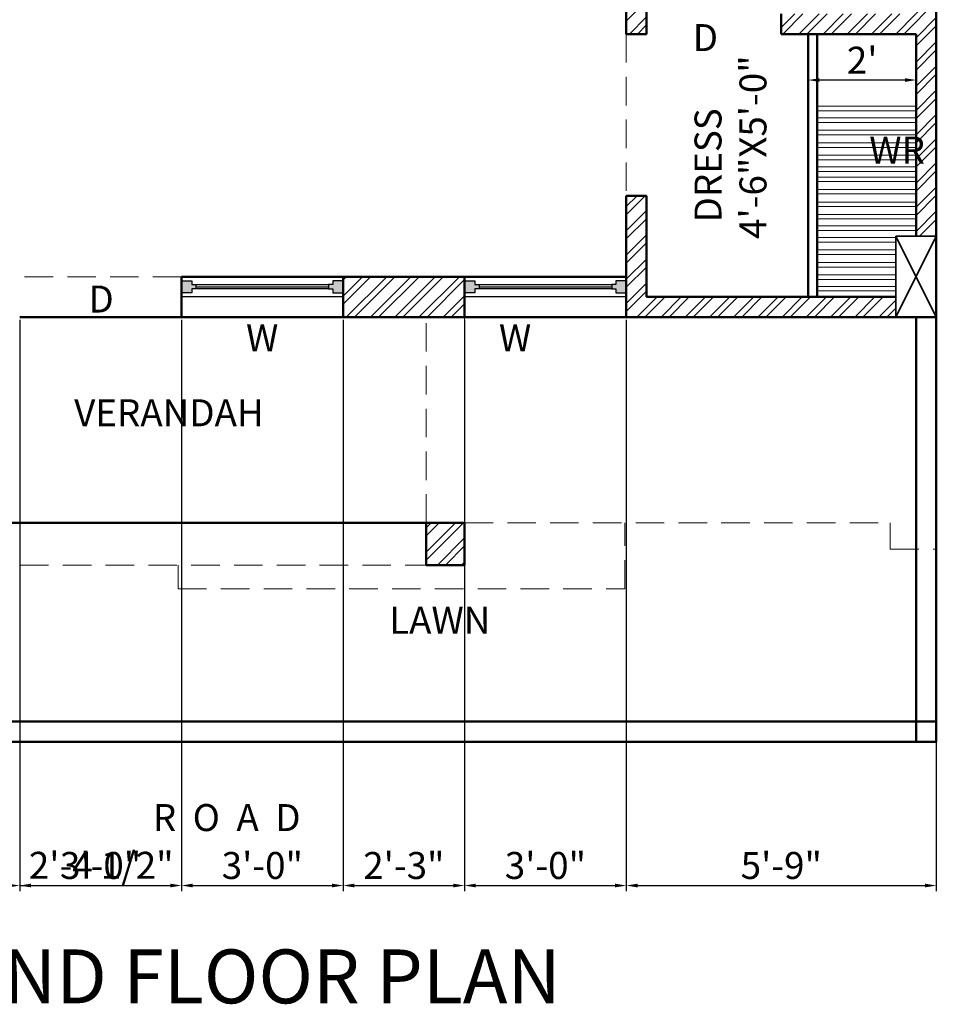
# Model space of a CAD drawing. Units: millimetres. Extents: x 67033 to 68301, y 155969 to 157209.
# Tile 2 of 17: x 67203 to 67407, y 156470 to 156689. Entities that reach past the tile are written whole.
import ezdxf

# ---------------------------------------------------------------- set-up
doc = ezdxf.new("R2010")
doc.units = ezdxf.units.MM
doc.linetypes.add('HIDDEN', pattern=[9.525, 6.35, -3.175])
for name, color, linetype, lineweight in [('A-ANNO-DIMS', 2, 'Continuous', 18), ('A-ANNO-TEXT', 7, 'Continuous', 18), ('A-AREA-IDEN', 3, 'Continuous', 18), ('A-COLS', 3, 'Continuous', 35), ('A-FLOR-OVHD', 1, 'HIDDEN', 18), ('A-FURN', 8, 'Continuous', 18), ('A-GLAZ', 4, 'Continuous', 25), ('A-WALL', 7, 'Continuous', 50), ('A-WALL-PATT', 8, 'Continuous', 13)]:
    doc.layers.add(name, color=color, linetype=linetype, lineweight=lineweight)
doc.styles.get("Standard").update_dxf_attribs({"font": 'arial.ttf'})
doc.dimstyles.new('ISO-25', dxfattribs={"dimtxt": 6, "dimasz": 2.5, "dimexe": 1.25, "dimexo": 0.625, "dimtad": 1, "dimdec": 0, "dimlunit": 3, "dimtxsty": 'Standard', "dimcen": 2.5, "dimadec": 0, "dimazin": 0, "dimtfac": 1, "dimtdec": 0, "dimtmove": 0, "dimatfit": 3, "dimfxl": 1, "dimarcsym": 0})

# ---------------------------------------------------------------- blocks, each defined once
blk = doc.blocks.new('*D26')
at = {"layer": 'A-ANNO-DIMS', "color": 0, "lineweight": -2, "transparency": 16777216}
for p, q in [((67378.94, 156675.41), (67378.94, 156674.01)), ((67400.44, 156675.26), (67381.44, 156675.26)), ((67402.94, 156675.41), (67402.94, 156674.01))]:
    blk.add_line(p, q, dxfattribs=at)
at = {"layer": 'A-ANNO-DIMS', "color": 0, "transparency": 16777216}
for points in [[(67381.44, 156675.67), (67381.44, 156674.84), (67378.94, 156675.26)], [(67400.44, 156675.67), (67400.44, 156674.84), (67402.94, 156675.26)]]:
    blk.add_solid(points, dxfattribs=at)
at = {"layer": 'Defpoints', "color": 0, "transparency": 16777216}
for p in [(67378.94, 156676.04), (67378.94, 156675.26), (67402.94, 156676.04)]:
    blk.add_point(p, dxfattribs=at)
at = {"layer": 'A-ANNO-DIMS', "color": 0, "transparency": 16777216, "insert": (67390.94, 156678.89), "char_height": 6, "attachment_point": 5}
blk.add_mtext("2'", dxfattribs=at)
blk = doc.blocks.new('WIN-900')
for p, q in [((3.67, 3.22), (33.2, 3.22)), ((3.67, 2.74), (33.2, 2.74)), ((33.2, 2.27), (3.67, 2.27))]:
    blk.add_line(p, q)
blk.add_lwpolyline([(0.44, 4.99), (36.44, 4.99), (36.44, 0.49), (0.44, 0.49)], close=True)
for points in [[(0.44, 4.09), (2.73, 4.09), (2.73, 3.22), (3.67, 3.22), (3.67, 2.27), (2.73, 2.27), (2.73, 1.4), (0.44, 1.4)], [(36.44, 4.09), (34.14, 4.09), (34.14, 3.22), (33.2, 3.22), (33.2, 2.27), (34.14, 2.27), (34.14, 1.4), (36.44, 1.4)]]:
    blk.add_lwpolyline(points)
blk = doc.blocks.new('COLUMN-230x460')
for p, q in [((0.44, 17.99), (9.44, -0.01)), ((9.44, 17.99), (0.44, -0.01))]:
    blk.add_line(p, q)
blk.add_lwpolyline([(0.44, 17.99), (9.44, 17.99), (9.44, -0.01), (0.44, -0.01)], close=True)
blk = doc.blocks.new('*D87')
at = {"layer": 'A-ANNO-DIMS', "color": 0, "lineweight": -2, "transparency": 16777216}
for p, q in [((67174.94, 156621.87), (67174.94, 156494.74)), ((67203.44, 156621.87), (67203.44, 156494.74)), ((67177.44, 156495.99), (67200.94, 156495.99)), ((67203.44, 156495.99), (67237.22, 156495.99))]:
    blk.add_line(p, q, dxfattribs=at)
at = {"layer": 'A-ANNO-DIMS', "color": 0, "transparency": 16777216}
for points in [[(67177.44, 156496.41), (67177.44, 156495.58), (67174.94, 156495.99)], [(67200.94, 156496.41), (67200.94, 156495.58), (67203.44, 156495.99)]]:
    blk.add_solid(points, dxfattribs=at)
at = {"layer": 'Defpoints', "color": 0, "transparency": 16777216}
for p in [(67174.94, 156622.49), (67203.44, 156622.49), (67203.44, 156495.99)]:
    blk.add_point(p, dxfattribs=at)
at = {"layer": 'A-ANNO-DIMS', "color": 0, "transparency": 16777216, "insert": (67221.58, 156499.72), "char_height": 6, "attachment_point": 5}
blk.add_mtext('2\'-4 1/2"', dxfattribs=at)
blk = doc.blocks.new('*D88')
at = {"layer": 'A-ANNO-DIMS', "color": 0, "lineweight": -2, "transparency": 16777216}
for p, q in [((67203.44, 156621.87), (67203.44, 156494.74)), ((67239.44, 156621.87), (67239.44, 156494.74)), ((67205.94, 156495.99), (67236.94, 156495.99))]:
    blk.add_line(p, q, dxfattribs=at)
at = {"layer": 'A-ANNO-DIMS', "color": 0, "transparency": 16777216}
for points in [[(67205.94, 156496.41), (67205.94, 156495.58), (67203.44, 156495.99)], [(67236.94, 156496.41), (67236.94, 156495.58), (67239.44, 156495.99)]]:
    blk.add_solid(points, dxfattribs=at)
at = {"layer": 'Defpoints', "color": 0, "transparency": 16777216}
for p in [(67203.44, 156622.49), (67239.44, 156622.49), (67239.44, 156495.99)]:
    blk.add_point(p, dxfattribs=at)
at = {"layer": 'A-ANNO-DIMS', "color": 0, "transparency": 16777216, "insert": (67221.44, 156499.68), "char_height": 6, "attachment_point": 5}
blk.add_mtext('3\'-0"', dxfattribs=at)
blk = doc.blocks.new('*D89')
at = {"layer": 'A-ANNO-DIMS', "color": 0, "lineweight": -2, "transparency": 16777216}
for p, q in [((67239.44, 156621.87), (67239.44, 156494.74)), ((67275.44, 156621.87), (67275.44, 156494.74)), ((67241.94, 156495.99), (67272.94, 156495.99))]:
    blk.add_line(p, q, dxfattribs=at)
at = {"layer": 'A-ANNO-DIMS', "color": 0, "transparency": 16777216}
for points in [[(67241.94, 156496.41), (67241.94, 156495.58), (67239.44, 156495.99)], [(67272.94, 156496.41), (67272.94, 156495.58), (67275.44, 156495.99)]]:
    blk.add_solid(points, dxfattribs=at)
at = {"layer": 'Defpoints', "color": 0, "transparency": 16777216}
for p in [(67239.44, 156622.49), (67275.44, 156622.49), (67275.44, 156495.99)]:
    blk.add_point(p, dxfattribs=at)
at = {"layer": 'A-ANNO-DIMS', "color": 0, "transparency": 16777216, "insert": (67257.44, 156499.68), "char_height": 6, "attachment_point": 5}
blk.add_mtext('3\'-0"', dxfattribs=at)
blk = doc.blocks.new('*D90')
at = {"layer": 'A-ANNO-DIMS', "color": 0, "lineweight": -2, "transparency": 16777216}
for p, q in [((67275.44, 156621.87), (67275.44, 156494.74)), ((67302.44, 156621.87), (67302.44, 156494.74)), ((67277.94, 156495.99), (67299.94, 156495.99))]:
    blk.add_line(p, q, dxfattribs=at)
at = {"layer": 'A-ANNO-DIMS', "color": 0, "transparency": 16777216}
for points in [[(67277.94, 156496.41), (67277.94, 156495.58), (67275.44, 156495.99)], [(67299.94, 156496.41), (67299.94, 156495.58), (67302.44, 156495.99)]]:
    blk.add_solid(points, dxfattribs=at)
at = {"layer": 'Defpoints', "color": 0, "transparency": 16777216}
for p in [(67275.44, 156622.49), (67302.44, 156622.49), (67302.44, 156495.99)]:
    blk.add_point(p, dxfattribs=at)
at = {"layer": 'A-ANNO-DIMS', "color": 0, "transparency": 16777216, "insert": (67288.94, 156499.68), "char_height": 6, "attachment_point": 5}
blk.add_mtext('2\'-3"', dxfattribs=at)
blk = doc.blocks.new('*D91')
at = {"layer": 'A-ANNO-DIMS', "color": 0, "lineweight": -2, "transparency": 16777216}
for p, q in [((67302.44, 156621.87), (67302.44, 156494.74)), ((67338.44, 156621.87), (67338.44, 156494.74)), ((67304.94, 156495.99), (67335.94, 156495.99))]:
    blk.add_line(p, q, dxfattribs=at)
at = {"layer": 'A-ANNO-DIMS', "color": 0, "transparency": 16777216}
for points in [[(67304.94, 156496.41), (67304.94, 156495.58), (67302.44, 156495.99)], [(67335.94, 156496.41), (67335.94, 156495.58), (67338.44, 156495.99)]]:
    blk.add_solid(points, dxfattribs=at)
at = {"layer": 'Defpoints', "color": 0, "transparency": 16777216}
for p in [(67302.44, 156622.49), (67338.44, 156622.49), (67338.44, 156495.99)]:
    blk.add_point(p, dxfattribs=at)
at = {"layer": 'A-ANNO-DIMS', "color": 0, "transparency": 16777216, "insert": (67320.44, 156499.68), "char_height": 6, "attachment_point": 5}
blk.add_mtext('3\'-0"', dxfattribs=at)
blk = doc.blocks.new('*D92')
at = {"layer": 'A-ANNO-DIMS', "color": 0, "lineweight": -2, "transparency": 16777216}
for p, q in [((67338.44, 156621.87), (67338.44, 156494.74)), ((67407.44, 156621.87), (67407.44, 156494.74)), ((67340.94, 156495.99), (67404.94, 156495.99))]:
    blk.add_line(p, q, dxfattribs=at)
at = {"layer": 'A-ANNO-DIMS', "color": 0, "transparency": 16777216}
for points in [[(67340.94, 156496.41), (67340.94, 156495.58), (67338.44, 156495.99)], [(67404.94, 156496.41), (67404.94, 156495.58), (67407.44, 156495.99)]]:
    blk.add_solid(points, dxfattribs=at)
at = {"layer": 'Defpoints', "color": 0, "transparency": 16777216}
for p in [(67338.44, 156622.49), (67407.44, 156622.49), (67407.44, 156495.99)]:
    blk.add_point(p, dxfattribs=at)
at = {"layer": 'A-ANNO-DIMS', "color": 0, "transparency": 16777216, "insert": (67372.94, 156499.68), "char_height": 6, "attachment_point": 5}
blk.add_mtext('5\'-9"', dxfattribs=at)

msp = doc.modelspace()

# ---------------------------------------------------------------- hatches: boundary and pattern name
at = {"layer": 'A-GLAZ'}
h = msp.add_hatch(color=256, dxfattribs=at)
h.dxf.hatch_style = 1
h.paths.add_polyline_path([(67241.73, 156628.77), (67242.67, 156628.77), (67242.67, 156629.72), (67241.73, 156629.72), (67241.73, 156630.59), (67239.44, 156630.59), (67239.44, 156627.9), (67241.73, 156627.9)], flags=17)
h = msp.add_hatch(color=256, dxfattribs=at)
h.dxf.hatch_style = 1
h.paths.add_polyline_path([(67275.44, 156630.59), (67273.14, 156630.59), (67273.14, 156629.72), (67272.2, 156629.72), (67272.2, 156628.77), (67273.14, 156628.77), (67273.14, 156627.9), (67275.44, 156627.9)])
h = msp.add_hatch(color=256, dxfattribs=at)
h.dxf.hatch_style = 1
h.paths.add_polyline_path([(67305.67, 156629.72), (67304.73, 156629.72), (67304.73, 156630.59), (67302.44, 156630.59), (67302.44, 156627.9), (67304.73, 156627.9), (67304.73, 156628.77), (67305.67, 156628.77)])
h = msp.add_hatch(color=256, dxfattribs=at)
h.dxf.hatch_style = 1
h.paths.add_polyline_path([(67338.44, 156630.59), (67336.14, 156630.59), (67336.14, 156629.72), (67335.2, 156629.72), (67335.2, 156628.77), (67336.14, 156628.77), (67336.14, 156627.9), (67338.44, 156627.9)])
at = {"layer": 'A-WALL-PATT'}
h = msp.add_hatch(dxfattribs=at)
h.set_pattern_fill('ANSI32', color=256, scale=0.4)
h.paths.add_polyline_path([(67407.44, 156941.99), (67402.94, 156941.99), (67402.94, 156802.49), (67342.94, 156802.49), (67342.94, 156822.09), (67342.94, 156871.49), (67338.44, 156871.49), (67338.44, 156770.99), (67236.44, 156770.99), (67236.44, 156766.49), (67338.44, 156766.49), (67338.44, 156685.49), (67342.94, 156685.49), (67342.94, 156797.99), (67402.94, 156797.99), (67402.94, 156767.19), (67407.44, 156767.19)])
h = msp.add_hatch(dxfattribs=at)
h.set_pattern_fill('ANSI32', color=256, scale=0.4)
h.paths.add_polyline_path([(67407.44, 156749.19), (67402.94, 156749.19), (67402.94, 156689.99), (67384.62, 156689.99), (67372.94, 156689.99), (67372.94, 156685.49), (67402.94, 156685.49), (67402.94, 156640.49), (67407.44, 156640.49)])
h = msp.add_hatch(dxfattribs=at)
h.set_pattern_fill('ANSI32', color=256, scale=0.4)
h.paths.add_polyline_path([(67398.44, 156626.99), (67342.94, 156626.99), (67342.94, 156649.49), (67338.44, 156649.49), (67338.44, 156622.49), (67398.44, 156622.49)])
h = msp.add_hatch(dxfattribs=at)
h.set_pattern_fill('ANSI32', color=256, scale=0.4)
h.paths.add_polyline_path([(67302.44, 156631.49), (67275.44, 156631.49), (67275.44, 156626.99), (67275.44, 156622.49), (67302.44, 156622.49)])
h = msp.add_hatch(dxfattribs=at)
h.set_pattern_fill('ANSI32', color=256, scale=0.4)
h.paths.add_polyline_path([(67302.44, 156576.72), (67293.89, 156576.72), (67293.89, 156567.32), (67302.44, 156567.32)])

# ---------------------------------------------------------------- linework, layer by layer
at = {"layer": 'A-FLOR-OVHD'}
for p, q in [((67338.44, 156685.49), (67338.44, 156649.49)), ((67239.44, 156631.49), (67203.44, 156631.49)), ((67293.89, 156576.72), (67293.89, 156622.49)), ((67302.44, 156622.49), (67302.44, 156567.32)), ((67302.44, 156576.72), (67397.18, 156576.72)), ((67338.08, 156562.05), (67338.08, 156576.72)), ((67397.18, 156576.72), (67397.18, 156570.83)), ((67397.18, 156570.83), (67407.44, 156570.83)), ((67174.94, 156567.32), (67302.44, 156567.32)), ((67238.69, 156567.32), (67238.69, 156562.05)), ((67238.69, 156562.05), (67338.08, 156562.05))]:
    msp.add_line(p, q, dxfattribs=at)
at = {"layer": 'A-FURN'}
for p, q in [((67380.94, 156669.41), (67402.94, 156669.41)), ((67380.94, 156668.41), (67402.94, 156668.41)), ((67380.94, 156666.82), (67402.94, 156666.82)), ((67380.94, 156665.82), (67402.94, 156665.82)), ((67380.94, 156664.09), (67402.94, 156664.09)), ((67380.94, 156663.09), (67402.94, 156663.09)), ((67380.94, 156661.27), (67402.94, 156661.27)), ((67380.94, 156660.27), (67402.94, 156660.27)), ((67380.94, 156658.53), (67402.94, 156658.53)), ((67380.94, 156657.53), (67402.94, 156657.53)), ((67380.94, 156655.94), (67402.94, 156655.94)), ((67380.94, 156654.94), (67402.94, 156654.94)), ((67380.94, 156653.66), (67402.94, 156653.66)), ((67380.94, 156652.66), (67402.94, 156652.66)), ((67380.94, 156650.92), (67402.94, 156650.92)), ((67380.94, 156649.92), (67402.94, 156649.92)), ((67380.94, 156648.11), (67402.94, 156648.11)), ((67380.94, 156647.11), (67402.94, 156647.11)), ((67380.94, 156645.36), (67402.94, 156645.36)), ((67380.94, 156644.36), (67402.94, 156644.36)), ((67380.94, 156642.78), (67402.94, 156642.78)), ((67380.94, 156641.78), (67402.94, 156641.78)), ((67380.94, 156640.19), (67398.44, 156640.19)), ((67380.94, 156639.19), (67398.44, 156639.19)), ((67380.94, 156637.46), (67398.44, 156637.46)), ((67380.94, 156636.46), (67398.44, 156636.46)), ((67380.94, 156634.64), (67398.44, 156634.64)), ((67380.94, 156633.64), (67398.44, 156633.64)), ((67380.94, 156631.9), (67398.44, 156631.9)), ((67380.94, 156630.9), (67398.44, 156630.9)), ((67380.94, 156629.31), (67398.44, 156629.31)), ((67380.94, 156628.31), (67398.44, 156628.31))]:
    msp.add_line(p, q, dxfattribs=at)
at = {"layer": 'A-WALL'}
for p, q in [((67407.44, 157140.99), (67407.44, 156527.99)), ((67342.94, 156797.99), (67342.94, 156685.49)), ((67338.44, 156766.49), (67338.44, 156685.49)), ((67372.94, 156689.99), (67372.94, 156685.49)), ((67338.44, 156685.49), (67342.94, 156685.49)), ((67372.94, 156685.49), (67402.94, 156685.49)), ((67378.94, 156685.49), (67378.94, 156626.99)), ((67380.94, 156685.49), (67380.94, 156626.99)), ((67402.94, 156685.49), (67402.94, 156640.49)), ((67338.44, 156649.49), (67342.94, 156649.49)), ((67338.44, 156649.49), (67338.44, 156622.49)), ((67342.94, 156649.49), (67342.94, 156626.99)), ((67239.44, 156631.49), (67239.44, 156622.49)), ((67239.44, 156631.49), (67338.44, 156631.49)), ((67239.44, 156631.49), (67239.44, 156626.99)), ((67275.44, 156631.49), (67275.44, 156622.49)), ((67275.44, 156631.49), (67275.44, 156626.99)), ((67302.44, 156631.49), (67302.44, 156622.49)), ((67302.44, 156631.49), (67302.44, 156626.99)), ((67338.44, 156631.49), (67338.44, 156626.99)), ((67342.94, 156626.99), (67398.44, 156626.99)), ((67203.44, 156622.49), (67239.44, 156622.49)), ((67239.44, 156622.49), (67407.44, 156622.49)), ((67402.94, 156622.49), (67402.94, 156527.99)), ((67174.94, 156576.72), (67302.44, 156576.72)), ((67192.94, 156532.49), (67407.44, 156532.49)), ((67068.44, 156527.99), (67407.44, 156527.99))]:
    msp.add_line(p, q, dxfattribs=at)
msp.add_lwpolyline([(67293.89, 156567.32), (67302.44, 156567.32), (67302.44, 156576.72), (67293.89, 156576.72)], close=True, dxfattribs=at)

# ---------------------------------------------------------------- block references
at = {"layer": 'A-COLS', "rotation": 180}
msp.add_blockref('COLUMN-230x460', (67407.87, 156640.49), dxfattribs=at)
at = {"layer": 'A-GLAZ'}
for p in [(67239, 156626.5), (67302, 156626.5)]:
    msp.add_blockref('WIN-900', p, dxfattribs=at)

# ---------------------------------------------------------------- texts
at = {"layer": 'A-ANNO-TEXT', "attachment_point": 1}
for s, width, insert, char_height in [('   D', 19.5287, (67347.73, 156687.7), 6), ('   WR', 19.5287, (67387.01, 156662.68), 6), ('   D', 19.5287, (67213.24, 156629.51), 6), ('   W', 19.5287, (67248.32, 156620.89), 6), ('   W', 19.5287, (67304.6, 156620.88), 6), ('GROUND FLOOR PLAN', 203.6887, (67154.11, 156481.77), 12)]:
    msp.add_mtext_dynamic_manual_height_columns(s, width=width, gutter_width=12.5, heights=[0], dxfattribs=dict(at, insert=insert, char_height=char_height))
at = {"layer": 'A-AREA-IDEN', "insert": (67353.63, 156638.06), "char_height": 6, "attachment_point": 1, "rotation": 90}
msp.add_mtext_dynamic_manual_height_columns('   DRESS\\P 4\'-6"X5\'-0"', width=46.8836, gutter_width=12.5, heights=[0], dxfattribs=at)
at = {"layer": 'A-AREA-IDEN', "char_height": 6, "attachment_point": 1}
for s, insert in [('   VERANDAH', (67210.06, 156604.2)), ('   LAWN', (67280.16, 156558.02)), ('   R  O  A  D', (67227.57, 156514.12))]:
    msp.add_mtext_dynamic_manual_height_columns(s, width=59.4046, gutter_width=12.5, heights=[0], dxfattribs=dict(at, insert=insert))

# ---------------------------------------------------------------- dimensions: what is measured, and where the dimension line sits
at = {"layer": 'A-ANNO-DIMS'}
for base, p1, p2, override, picture, middle in [((67378.94, 156675.26), (67402.94, 156676.04), (67378.94, 156676.04), {"dimclrd": 0, "dimclre": 0, "dimclrt": 0}, '*D26', (67390.94, 156678.89)), ((67203.44, 156495.99), (67174.94, 156622.49), (67203.44, 156622.49), {"dimdec": 1, "dimlfac": 1, "dimrnd": 0, "dimzin": 1, "dimdsep": 46, "dimlunit": 4, "dimfrac": 2}, '*D87', (67221.58, 156499.72)), ((67239.44, 156495.99), (67203.44, 156622.49), (67239.44, 156622.49), {"dimdec": 1, "dimlfac": 1, "dimrnd": 0, "dimzin": 1, "dimdsep": 46, "dimlunit": 4, "dimfrac": 2}, '*D88', (67221.44, 156499.68)), ((67275.44, 156495.99), (67239.44, 156622.49), (67275.44, 156622.49), {"dimdec": 1, "dimlfac": 1, "dimrnd": 0, "dimzin": 1, "dimdsep": 46, "dimlunit": 4, "dimfrac": 2}, '*D89', (67257.44, 156499.68)), ((67302.44, 156495.99), (67275.44, 156622.49), (67302.44, 156622.49), {"dimdec": 1, "dimlfac": 1, "dimrnd": 0, "dimzin": 1, "dimdsep": 46, "dimlunit": 4, "dimfrac": 2}, '*D90', (67288.94, 156499.68)), ((67338.44, 156495.99), (67302.44, 156622.49), (67338.44, 156622.49), {"dimdec": 1, "dimlfac": 1, "dimrnd": 0, "dimzin": 1, "dimdsep": 46, "dimlunit": 4, "dimfrac": 2}, '*D91', (67320.44, 156499.68)), ((67407.44, 156495.99), (67338.44, 156622.49), (67407.44, 156622.49), {"dimdec": 1, "dimlfac": 1, "dimrnd": 0, "dimzin": 1, "dimdsep": 46, "dimlunit": 4, "dimfrac": 2}, '*D92', (67372.94, 156499.68))]:
    dim = msp.add_linear_dim(base=base, p1=p1, p2=p2, dimstyle='ISO-25', override=override, dxfattribs=at)
    dim.commit()
    dim.dimension.update_dxf_attribs({"geometry": picture, "text_midpoint": middle})

doc.saveas('drawing.dxf')
